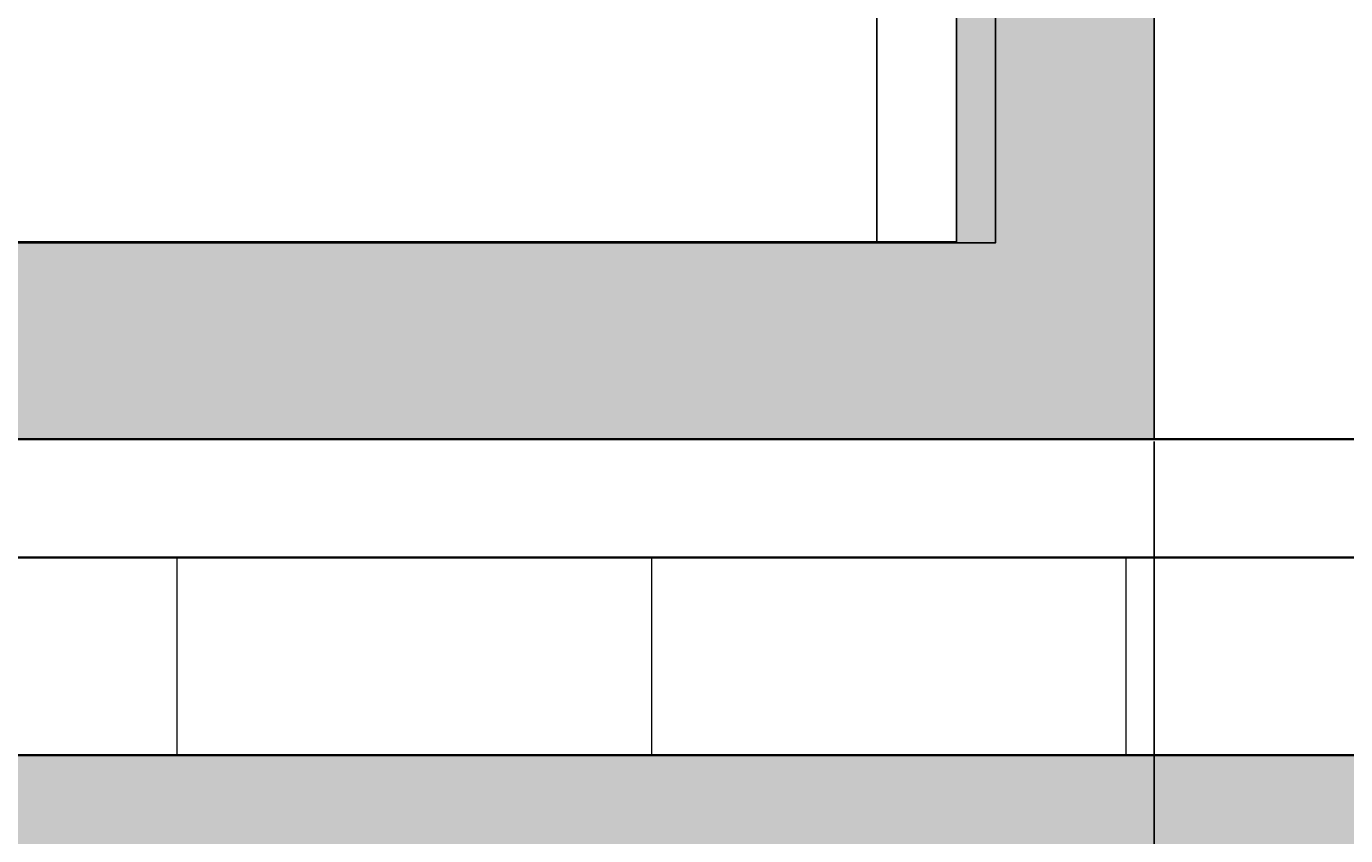
# Model space of a CAD drawing. Units: inches. Extents: x -301 to 715, y -607 to 364.
# Tile 22 of 141: x -16 to 18, y -474 to -453. Entities that reach past the tile are written whole.
import ezdxf

# ---------------------------------------------------------------- set-up
doc = ezdxf.new("R2010")
doc.units = ezdxf.units.IN
doc.header["$MEASUREMENT"] = 0
for name, color, linetype, lineweight in [('A-ANNO-DIMS', 2, 'Continuous', 18), ('A-DOOR', 4, 'Continuous', 25), ('A-SECT', 1, 'Continuous', 35), ('A-SECT-PATT', 8, 'Continuous', 13)]:
    doc.layers.add(name, color=color, linetype=linetype, lineweight=lineweight)
doc.styles.get("Standard").update_dxf_attribs({"font": 'arial.ttf'})
doc.dimstyles.get("Standard").update_dxf_attribs({"dimtxt": 0.18, "dimasz": 0.18, "dimexe": 0.18, "dimexo": 0.0625, "dimgap": 0.09, "dimtad": 0, "dimtih": 1, "dimtoh": 1, "dimdec": 1, "dimzin": 0, "dimdsep": 46, "dimlunit": 4, "dimtxsty": 'Standard', "dimcen": 0.09, "dimclrd": 3, "dimclre": 4, "dimclrt": 6, "dimadec": 0, "dimazin": 0, "dimtfac": 1, "dimtdec": 1, "dimtofl": 0, "dimtmove": 0, "dimatfit": 3, "dimfxl": 1, "dimtfill": 2, "dimtfillclr": 51, "dimtolj": 1, "dimtzin": 0, "dimarcsym": 0})

# ---------------------------------------------------------------- blocks, each defined once
blk = doc.blocks.new('*U75')
blk.add_lwpolyline([(3.124, 0.013), (0.124, 0.013), (0.124, 72.013), (40.124, 72.013), (40.124, 0.013), (37.124, 0.013)])
blk.add_lwpolyline([(37.124, 68.99), (37.124, 0.013), (3.124, 0.013), (3.124, 68.99)], close=True)
blk = doc.blocks.new('*D176')
at = {"layer": 'A-ANNO-DIMS', "color": 4, "lineweight": -2, "transparency": 16777216}
for p, q in [((148.28, -324.477), (215.605, -324.477)), ((-15.22, -540.477), (215.605, -540.477))]:
    blk.add_line(p, q, dxfattribs=at)
at = {"layer": 'A-ANNO-DIMS', "color": 3, "lineweight": -2, "transparency": 16777216}
for p, q in [((215.425, -324.657), (215.425, -432.296)), ((215.425, -540.297), (215.425, -432.659))]:
    blk.add_line(p, q, dxfattribs=at)
at = {"layer": 'A-ANNO-DIMS', "color": 3, "transparency": 16777216}
for points in [[(215.395, -324.657), (215.455, -324.657), (215.425, -324.477)], [(215.395, -540.297), (215.455, -540.297), (215.425, -540.477)]]:
    blk.add_solid(points, dxfattribs=at)
at = {"layer": 'Defpoints', "color": 0, "transparency": 16777216}
for p in [(148.218, -324.477), (-15.282, -540.477), (215.425, -540.477)]:
    blk.add_point(p, dxfattribs=at)
at = {"layer": 'A-ANNO-DIMS', "color": 6, "transparency": 16777216, "insert": (215.425, -432.477), "char_height": 0.18, "attachment_point": 5, "bg_fill": 1, "box_fill_scale": 1.25, "bg_fill_color": 51, "bg_fill_transparency": 0}
blk.add_mtext('\\A1;18\'-0"', dxfattribs=at)
blk = doc.blocks.new('*D180')
at = {"layer": 'A-ANNO-DIMS', "color": 4, "lineweight": -2, "transparency": 16777216}
for p, q in [((-35.282, -463.54), (-35.282, -573.809)), ((12.718, -463.54), (12.718, -573.809))]:
    blk.add_line(p, q, dxfattribs=at)
at = {"layer": 'A-ANNO-DIMS', "color": 3, "lineweight": -2, "transparency": 16777216}
for p, q in [((-35.102, -573.629), (-11.615, -573.629)), ((12.538, -573.629), (-10.949, -573.629))]:
    blk.add_line(p, q, dxfattribs=at)
at = {"layer": 'A-ANNO-DIMS', "color": 3, "transparency": 16777216}
for points in [[(-35.102, -573.599), (-35.102, -573.659), (-35.282, -573.629)], [(12.538, -573.599), (12.538, -573.659), (12.718, -573.629)]]:
    blk.add_solid(points, dxfattribs=at)
at = {"layer": 'Defpoints', "color": 0, "transparency": 16777216}
for p in [(-35.282, -463.477), (12.718, -463.477), (12.718, -573.629)]:
    blk.add_point(p, dxfattribs=at)
at = {"layer": 'A-ANNO-DIMS', "color": 6, "transparency": 16777216, "insert": (-11.282, -573.629), "char_height": 0.18, "attachment_point": 5, "bg_fill": 1, "box_fill_scale": 1.25, "bg_fill_color": 51, "bg_fill_transparency": 0}
blk.add_mtext('\\A1;4\'-0"', dxfattribs=at)
blk = doc.blocks.new('*D181')
at = {"layer": 'A-ANNO-DIMS', "color": 4, "lineweight": -2, "transparency": 16777216}
for p, q in [((48.468, -433.54), (48.468, -573.809)), ((12.718, -463.54), (12.718, -573.809))]:
    blk.add_line(p, q, dxfattribs=at)
at = {"layer": 'A-ANNO-DIMS', "color": 3, "lineweight": -2, "transparency": 16777216}
for p, q in [((12.898, -573.629), (30.264, -573.629)), ((48.288, -573.629), (30.922, -573.629))]:
    blk.add_line(p, q, dxfattribs=at)
at = {"layer": 'A-ANNO-DIMS', "color": 3, "transparency": 16777216}
for points in [[(12.898, -573.599), (12.898, -573.659), (12.718, -573.629)], [(48.288, -573.599), (48.288, -573.659), (48.468, -573.629)]]:
    blk.add_solid(points, dxfattribs=at)
at = {"layer": 'Defpoints', "color": 0, "transparency": 16777216}
for p in [(48.468, -433.477), (12.718, -463.477), (48.468, -573.629)]:
    blk.add_point(p, dxfattribs=at)
at = {"layer": 'A-ANNO-DIMS', "color": 6, "transparency": 16777216, "insert": (30.593, -573.629), "char_height": 0.18, "attachment_point": 5, "bg_fill": 1, "box_fill_scale": 1.25, "bg_fill_color": 51, "bg_fill_transparency": 0}
blk.add_mtext('\\A1;3\'-0"', dxfattribs=at)

msp = doc.modelspace()

# ---------------------------------------------------------------- hatches: boundary and pattern name
at = {"layer": 'A-SECT-PATT'}
h = msp.add_hatch(dxfattribs=at)
h.set_pattern_fill('AR-CONC', color=256, scale=0.5)
h.set_pattern_definition([(50, (10.3213, 33.8764), (3.586301, -0.31376), [0.375, -4.125]), (355, (10.3213, 33.8764), (-0.693757, 3.76096), [0.3, -3.3]), (100.45144, (10.62, 33.8502), (2.892544, 3.4472), [0.3187, -3.50571]), (46.1842, (10.3213, 34.8764), (5.336207, -0.827596), [0.5625, -6.1875]), (96.6356, (10.766, 34.8074), (4.67331, 4.870593), [0.47805, -5.25857]), (351.1842, (10.321, 34.8764), (4.67331, 4.870593), [0.45, -4.95]), (21, (10.8213, 34.6264), (2.984535, -2.013094), [0.375, -4.125]), (326, (10.8213, 34.6264), (1.216577, 3.62575), [0.3, -3.3]), (71.45144, (11.07, 34.4586), (4.201112, 1.612656), [0.3187, -3.50571]), (37.5, (10.3213, 33.8764), (0.0607993, 1.6644693), [0, -3.26, 0, -3.35, 0, -3.3125]), (7.5, (10.3213, 33.8764), (1.3153477, 1.9720586), [0, -1.91, 0, -3.185, 0, -1.2625]), (327.5, (9.2063, 33.8764), (2.6691122, -0.1127744), [0, -1.25, 0, -3.9, 0, -5.175]), (317.5, (8.7063, 33.8764), (2.915931, 0.500525), [0, -1.625, 0, -2.59, 0, -3.675])])
h.paths.add_polyline_path([(-56.282, -535.477), (-61.282, -535.477), (-61.282, -540.477), (-15.282, -540.477), (-15.282, -535.477), (-20.282, -535.477)])
h.paths.add_polyline_path([(119.255, -535.477), (114.255, -535.477), (114.255, -540.477), (163.255, -540.477), (163.255, -535.477), (158.255, -535.477)])
h.paths.add_polyline_path([(-206.282, -471.477), (-209.282, -471.477), (-209.282, -481.477), (-206.282, -481.477), (-194.282, -481.477), (-194.282, -471.477)])
h.paths.add_polyline_path([(-41.282, -481.477), (-41.282, -471.477), (-185.282, -471.477), (-185.282, -481.477), (-180.282, -481.477)])
h.paths.add_polyline_path([(134.255, -481.477), (134.255, -471.477), (-35.282, -471.477), (-35.282, -481.477), (-30.282, -481.477)])
h.paths.add_polyline_path([(155.218, -481.477), (158.218, -481.477), (158.218, -471.477), (153.218, -471.477), (143.218, -471.477), (143.218, -481.477), (148.255, -481.477)])
h.paths.add_polyline_path([(-193.88, -356.477), (-193.904, -361.477), (143.218, -361.477), (143.218, -356.477)])
h = msp.add_hatch(color=256, dxfattribs=at)
h.dxf.hatch_style = 1
h.paths.add_polyline_path([(-138.282, -385.477), (-138.282, -433.477), (-87.981, -433.477), (-87.981, -385.477)])
h.paths.add_polyline_path([(-92.981, -390.477), (-92.981, -428.477), (-133.282, -428.477), (-133.282, -390.477)], flags=16)
h.paths.add_polyline_path([(-35.282, -385.477), (-35.282, -463.477), (12.718, -463.477), (12.718, -385.477)])
h.paths.add_polyline_path([(-30.282, -390.477), (7.718, -390.477), (7.718, -458.477), (-30.282, -458.477)], flags=16)
h.paths.add_polyline_path([(48.468, -385.477), (48.468, -433.477), (98.468, -433.477), (98.468, -385.477)])
h.paths.add_polyline_path([(93.468, -390.477), (93.468, -428.477), (53.468, -428.477), (53.468, -390.477)], flags=16)
h = msp.add_hatch(dxfattribs=at)
h.set_pattern_fill('ANSI31', color=256, scale=96, angle=45, style=0)
h.paths.add_polyline_path([(-35.282, -471.477), (134.255, -471.477), (134.255, -466.477), (-35.282, -466.477)])

# ---------------------------------------------------------------- linework, layer by layer
at = {"layer": 'A-DOOR'}
for points in [[(-35.282, -385.477), (12.718, -385.477), (12.718, -463.477), (-35.282, -463.477)], [(-30.282, -390.477), (7.718, -390.477), (7.718, -458.477), (-30.282, -458.477)]]:
    msp.add_lwpolyline(points, close=True, dxfattribs=at)
at = {"layer": 'A-SECT'}
for p, q in [((-199.282, -463.477), (148.255, -463.477)), ((-204.282, -466.477), (153.218, -466.477)), ((-206.282, -471.477), (155.218, -471.477))]:
    msp.add_line(p, q, dxfattribs=at)

# ---------------------------------------------------------------- block references
at = {"layer": 'A-DOOR'}
msp.add_blockref('*U75', (-31.421, -458.522), dxfattribs=at)

# ---------------------------------------------------------------- dimensions: what is measured, and where the dimension line sits
at = {"layer": 'A-ANNO-DIMS'}
dim = msp.add_linear_dim(base=(215.425, -540.477), p1=(148.218, -324.477), p2=(-15.282, -540.477), angle=90, dimstyle='Standard', override={"dimdec": 1, "dimlfac": 1, "dimrnd": 0, "dimzin": 1, "dimdsep": 46, "dimlunit": 4, "dimfrac": 2}, dxfattribs=at)
dim.commit()
dim.dimension.update_dxf_attribs({"geometry": '*D176', "text_midpoint": (215.425, -432.477)})
for base, p1, p2, picture, middle in [((48.467984, -573.628877), (12.717984, -463.47741), (48.467984, -433.47741), '*D181', (30.592984, -573.628877)), ((12.718, -573.629), (-35.282, -463.477), (12.718, -463.477), '*D180', (-11.282, -573.629))]:
    dim = msp.add_linear_dim(base=base, p1=p1, p2=p2, dimstyle='Standard', override={"dimdec": 1, "dimlfac": 1, "dimrnd": 0, "dimzin": 1, "dimdsep": 46, "dimlunit": 4, "dimfrac": 2}, dxfattribs=at)
    dim.commit()
    dim.dimension.update_dxf_attribs({"geometry": picture, "text_midpoint": middle})

doc.saveas('drawing.dxf')
